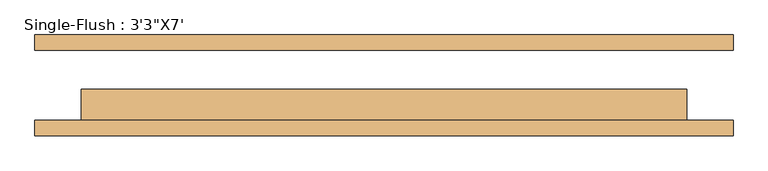
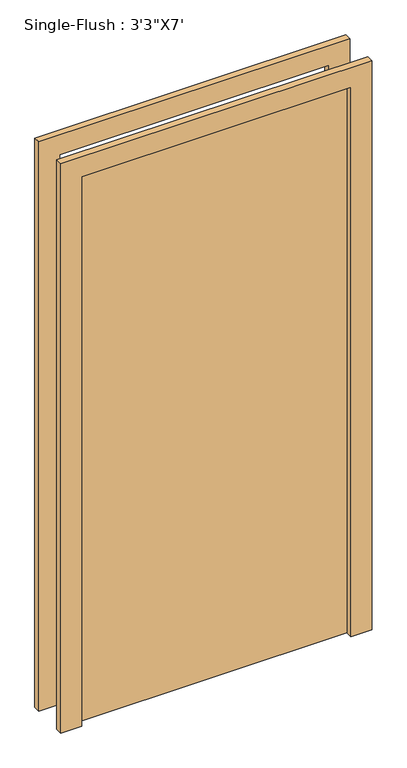
"""IFC4 building model written with IfcOpenShell, lengths in millimetres: door geometry."""

from ifc_helpers import new_model, si_unit, frame, origin, origin_with_axes, place, context, project, spatial, polyline, outline, extrude, source, transform, mapped, element, save


def door_43e5c869(model_context):
    return source(origin(), model_context, "Body", "SweptSolid", [
        extrude(outline(polyline([(2209.8, -571.5), (0.0, -571.5), (0.0, -495.3), (2133.6, -495.3), (2133.6, 495.3), (0.0, 495.3), (0.0, 571.5), (2209.8, 571.5), (2209.8, -571.5)])), frame((0.0, -82.55, 0.0), z_axis=(0.0, 1.0, 0.0), x_axis=(0.0, 0.0, 1.0)), (0.0, 0.0, 1.0), 25.4),
        extrude(outline(polyline([(2209.8, 571.5), (2209.8, -571.5), (0.0, -571.5), (0.0, -495.3), (2133.6, -495.3), (2133.6, 495.3), (0.0, 495.3), (0.0, 571.5), (2209.8, 571.5)])), frame((0.0, 57.15, 0.0), z_axis=(0.0, 1.0, 0.0), x_axis=(0.0, 0.0, 1.0)), (0.0, 0.0, 1.0), 25.4),
        extrude(outline(polyline([(495.3, -6.35), (495.3, -57.15), (-495.3, -57.15), (-495.3, -6.35), (495.3, -6.35)])), origin_with_axes(), (0.0, 0.0, 1.0), 2133.6),
    ])


if __name__ == "__main__":
    model = new_model("IFC4")
    model_context = context("Model", 3, world=origin())
    ifc_project = project(units=[si_unit("LENGTHUNIT", "METRE", prefix="MILLI")], contexts=[model_context])
    site = spatial("IfcSite", under=ifc_project)
    building = spatial("IfcBuilding", under=site)
    placement = place(None, origin())
    door_shape = door_43e5c869(model_context)
    element("IfcDoor", 1, ObjectType="Single-Flush : 3'3\"X7'", at=placement, inside=building, context=model_context, shape_type="MappedRepresentation", body=[
        mapped(door_shape, transform((0.0, 0.0, 0.0), x_axis=(1.0, 0.0, 0.0), y_axis=(0.0, 1.0, 0.0), z_axis=(0.0, 0.0, 1.0))),
    ])
    save(model, "model.ifc")

# Revit data of these elements
# Type "Single-Flush : 3'3\"X7'"
#   Type Mark = "11"
#   Construction Type Id = "MDOOR"
#   Assembly Code = "C1020"
#   Analytic Construction = "Metal"
#   Thickness = 0' - 2"
#   Heat Transfer Coefficient (U) = 0.651978 BTU/(h·ft²·°F)
#   Height = 7' - 0"
#   Trim Projection Ext = 0' - 1"
#   Trim Projection Int = 0' - 1"
#   Trim Width = 0' - 3"
#   Width = 3' - 3"
#   Define Thermal Properties by = 1
#   Door Material = Door - Panel
#   Frame Material = Door - Frame
#   Visual Light Transmittance = 0
#   Solar Heat Gain Coefficient = 0
#   Function = (empty or 0)
#   Wall Closure = (empty or 0)
# Element 1 (IfcDoor, "Single-Flush : 3'3\"X7'")
#   Materials on its faces: "Door - Frame", "Door - Panel"
# Materials
#   "Door - Panel": class "Wood", colour RGB 210 159 95, transparency 0, Cost = 0
#   "Door - Frame": colour RGB 118 70 51, transparency 0, Cost = 0
